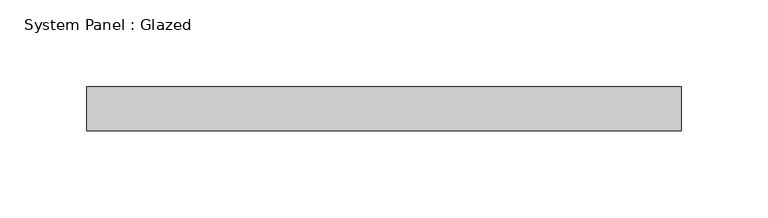
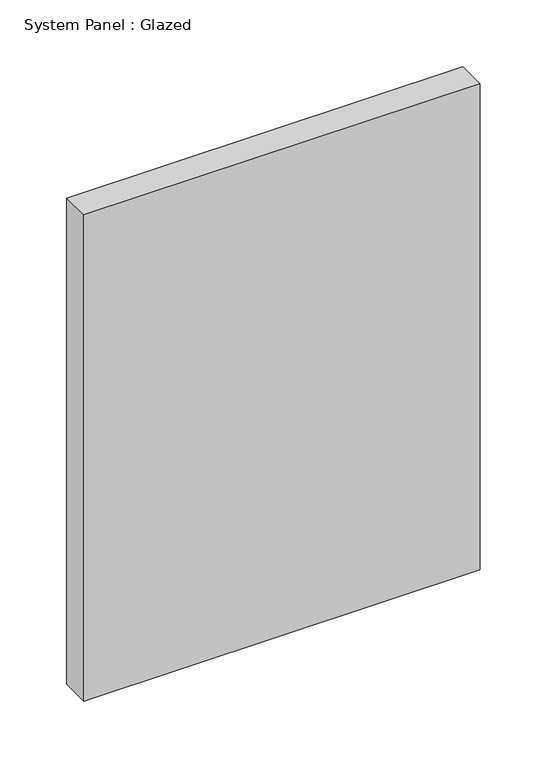
"""IFC4 building model written with IfcOpenShell, lengths in millimetres: plate geometry, System Panel : Glazed."""

from ifc_helpers import new_model, si_unit, origin, origin_with_axes, place, context, project, spatial, polyline, outline, extrude, source, transform, mapped, element, save


def system_panel_glazed_bfcc9025(model_context):
    return source(origin(), model_context, "Body", "SweptSolid", [
        extrude(outline(polyline([(171.45, 19.05), (-171.45, 19.05), (-171.45, 44.45), (171.45, 44.45), (171.45, 19.05)])), origin_with_axes(), (0.0, 0.0, 1.0), 444.5),
    ])


if __name__ == "__main__":
    model = new_model("IFC4")
    model_context = context("Model", 3, world=origin())
    ifc_project = project(units=[si_unit("LENGTHUNIT", "METRE", prefix="MILLI")], contexts=[model_context])
    site = spatial("IfcSite", under=ifc_project)
    building = spatial("IfcBuilding", under=site)
    placement = place(None, origin())
    system_panel_glazed_shape = system_panel_glazed_bfcc9025(model_context)
    element("IfcPlate", 1, ObjectType="System Panel : Glazed", at=placement, inside=building, context=model_context, shape_type="MappedRepresentation", body=[
        mapped(system_panel_glazed_shape, transform((0.0, 0.0, 0.0), x_axis=(1.0, 0.0, 0.0), y_axis=(0.0, 1.0, 0.0), z_axis=(0.0, 0.0, 1.0))),
    ])
    save(model, "model.ifc")

# Revit data of these elements
# Type "System Panel : Glazed"
#   Construction Type Id = "GSP4R"
#   Analytic Construction = "1/8 in Pilkington single glazing"
#   Visual Light Transmittance = 0.9
#   Solar Heat Gain Coefficient = 0.86
#   Heat Transfer Coefficient (U) = 1.18115 BTU/(h·ft²·°F)
#   Define Thermal Properties by = 1
# Element 1 (IfcPlate, "System Panel : Glazed")
#   Materials on its faces: "Glass"
# Materials
#   "Glass": class "Glass", colour RGB 0 128 192, transparency 0.75, Description = "Soda Lime Glass", Cost = 0
